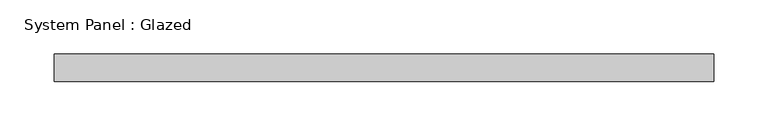
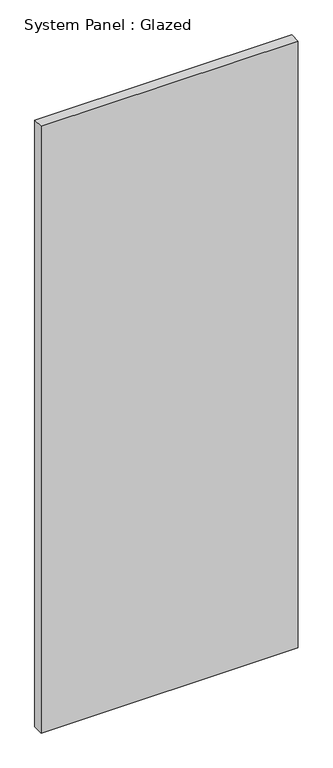
"""IFC4 building model written with IfcOpenShell, lengths in millimetres: plate geometry, System Panel : Glazed."""

from ifc_helpers import new_model, si_unit, origin, origin_with_axes, place, context, project, spatial, polyline, outline, extrude, source, transform, mapped, element, save


def system_panel_glazed_18e8007f(model_context):
    return source(origin(), model_context, "Body", "SweptSolid", [
        extrude(outline(polyline([(304.8, 19.05), (-304.8, 19.05), (-304.8, 44.45), (304.8, 44.45), (304.8, 19.05)])), origin_with_axes(), (0.0, 0.0, 1.0), 1519.9365008),
    ])


if __name__ == "__main__":
    model = new_model("IFC4")
    model_context = context("Model", 3, world=origin())
    ifc_project = project(units=[si_unit("LENGTHUNIT", "METRE", prefix="MILLI")], contexts=[model_context])
    site = spatial("IfcSite", under=ifc_project)
    building = spatial("IfcBuilding", under=site)
    placement = place(None, origin())
    system_panel_glazed_shape = system_panel_glazed_18e8007f(model_context)
    element("IfcPlate", 1, ObjectType="System Panel : Glazed", at=placement, inside=building, context=model_context, shape_type="MappedRepresentation", body=[
        mapped(system_panel_glazed_shape, transform((0.0, 0.0, 0.0), x_axis=(1.0, 0.0, 0.0), y_axis=(0.0, 1.0, 0.0), z_axis=(0.0, 0.0, 1.0))),
    ])
    save(model, "model.ifc")

# Revit data of these elements
# Type "System Panel : Glazed"
#   Construction Type Id = "GSP4R"
#   Analytic Construction = "1/8 in Pilkington single glazing"
#   Visual Light Transmittance = 0.9
#   Solar Heat Gain Coefficient = 0.86
#   Heat Transfer Coefficient (U) = 1.18115 BTU/(h·ft²·°F)
#   Define Thermal Properties by = 1
# Element 1 (IfcPlate, "System Panel : Glazed")
#   Materials on its faces: "Glass"
# Materials
#   "Glass": class "Glass", colour RGB 0 128 192, transparency 0.75, Description = "Soda Lime Glass", Cost = 0
